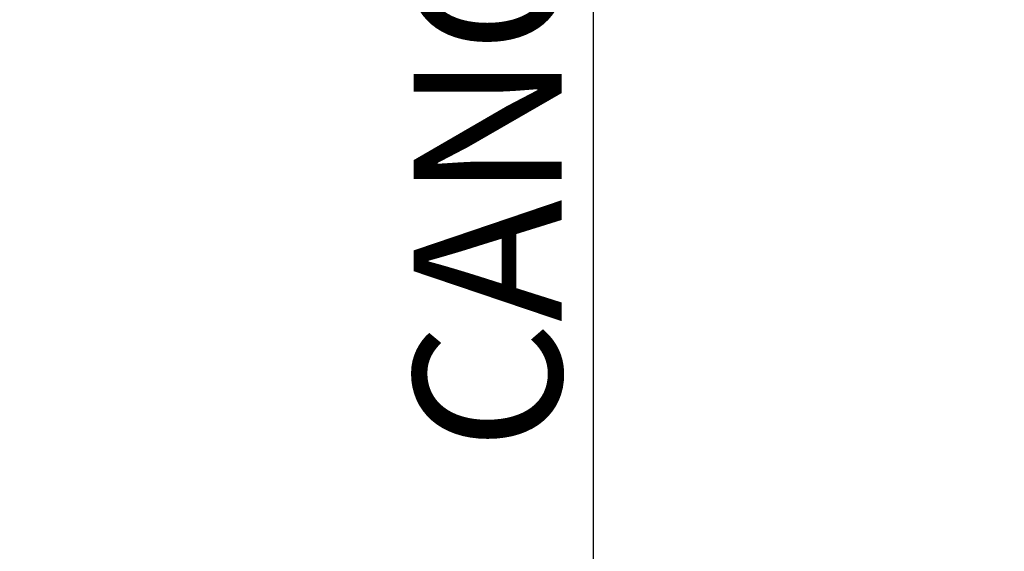
# Model space of a CAD drawing. Units: millimetres. Extents: x 595116 to 630915, y 909473 to 920225.
# Tile 65 of 134: x 629559 to 629619, y 919314 to 919346. Entities that reach past the tile are written whole.
import ezdxf

# ---------------------------------------------------------------- set-up
doc = ezdxf.new("R2010")
doc.units = ezdxf.units.MM
doc.layers.add('Dimension', color=3, linetype='Continuous', lineweight=18)
doc.styles.get("Standard").update_dxf_attribs({"font": 'arial.ttf'})
doc.dimstyles.new('ISO-25', dxfattribs={"dimtxt": 9, "dimasz": 6, "dimexe": 1.25, "dimexo": 0.625, "dimtad": 1, "dimlunit": 4, "dimtxsty": 'Standard', "dimcen": 2.5, "dimadec": 0, "dimazin": 0, "dimtfac": 1, "dimtmove": 0, "dimatfit": 3, "dimfxl": 1, "dimarcsym": 0})

# ---------------------------------------------------------------- blocks, each defined once
blk = doc.blocks.new('*D210')
at = {"layer": 'Defpoints', "color": 0, "transparency": 16777216}
for p in [(629586.227, 919310.123), (629593.946, 919310.123), (629586.227, 919258.662)]:
    blk.add_point(p, dxfattribs=at)
at = {"layer": 'Dimension', "color": 0, "lineweight": -2, "transparency": 16777216}
for p, q in [((629593.946, 919310.123), (629593.946, 919449.69)), ((629586.852, 919310.123), (629595.196, 919310.123)), ((629593.946, 919264.662), (629593.946, 919304.123)), ((629586.852, 919258.662), (629595.196, 919258.662))]:
    blk.add_line(p, q, dxfattribs=at)
at = {"layer": 'Dimension', "color": 0, "transparency": 16777216}
for points in [[(629592.946, 919304.123), (629594.946, 919304.123), (629593.946, 919310.123)], [(629592.946, 919264.662), (629594.946, 919264.662), (629593.946, 919258.662)]]:
    blk.add_solid(points, dxfattribs=at)
at = {"layer": 'Dimension', "color": 0, "transparency": 16777216, "insert": (629588.662, 919382.907), "char_height": 9, "attachment_point": 5, "rotation": 90}
blk.add_mtext('CANOPY 4\'-3 1/2" TYP.', dxfattribs=at)
blk = doc.blocks.new('*D216')
at = {"layer": 'Defpoints', "color": 0, "transparency": 16777216}
for p in [(629505.041, 919411.828), (629743.541, 919411.928), (629743.541, 918832.378)]:
    blk.add_point(p, dxfattribs=at)
at = {"layer": 'Dimension', "color": 0, "lineweight": -2, "transparency": 16777216}
for p, q in [((629505.041, 919411.203), (629505.041, 918831.128)), ((629743.541, 919411.303), (629743.541, 918831.128)), ((629511.041, 918832.378), (629737.541, 918832.378))]:
    blk.add_line(p, q, dxfattribs=at)
at = {"layer": 'Dimension', "color": 0, "transparency": 16777216}
for points in [[(629511.041, 918833.378), (629511.041, 918831.378), (629505.041, 918832.378)], [(629737.541, 918833.378), (629737.541, 918831.378), (629743.541, 918832.378)]]:
    blk.add_solid(points, dxfattribs=at)
at = {"layer": 'Dimension', "color": 0, "transparency": 16777216, "insert": (629624.291, 918837.656), "char_height": 9, "attachment_point": 5}
blk.add_mtext('19\'-10 1/2"', dxfattribs=at)
blk = doc.blocks.new('*D220')
at = {"layer": 'Defpoints', "color": 0, "transparency": 16777216}
for p in [(629824.951, 920160.756), (629511.274, 919302.009), (629824.951, 919302.009)]:
    blk.add_point(p, dxfattribs=at)
at = {"layer": 'Dimension', "color": 0, "lineweight": -2, "transparency": 16777216}
for p, q in [((629511.274, 919302.634), (629511.274, 920162.006)), ((629824.951, 919302.634), (629824.951, 920162.006)), ((629517.274, 920160.756), (629818.951, 920160.756))]:
    blk.add_line(p, q, dxfattribs=at)
at = {"layer": 'Dimension', "color": 0, "transparency": 16777216}
for points in [[(629517.274, 920161.756), (629517.274, 920159.756), (629511.274, 920160.756)], [(629818.951, 920161.756), (629818.951, 920159.756), (629824.951, 920160.756)]]:
    blk.add_solid(points, dxfattribs=at)
at = {"layer": 'Dimension', "color": 0, "transparency": 16777216, "insert": (629668.113, 920166.035), "char_height": 9, "attachment_point": 5}
blk.add_mtext('26\'-1 1/2"', dxfattribs=at)

msp = doc.modelspace()

# ---------------------------------------------------------------- dimensions: what is measured, and where the dimension line sits
at = {"layer": 'Dimension'}
for base, p1, p2, picture, middle in [((629824.951, 920160.756), (629511.274, 919302.009), (629824.951, 919302.009), '*D220', (629668.113, 920166.035)), ((629743.541, 918832.378), (629505.041, 919411.828), (629743.541, 919411.928), '*D216', (629624.291, 918837.656))]:
    dim = msp.add_linear_dim(base=base, p1=p1, p2=p2, dimstyle='ISO-25', override={"dimdec": 1, "dimlfac": 1, "dimrnd": 0, "dimzin": 1, "dimdsep": 46, "dimlunit": 4, "dimfrac": 2}, dxfattribs=at)
    dim.commit()
    dim.dimension.update_dxf_attribs({"geometry": picture, "text_midpoint": middle})
dim = msp.add_linear_dim(base=(629593.946, 919310.123), p1=(629586.227, 919258.662), p2=(629586.227, 919310.123), angle=90, text='CANOPY <> TYP.', dimstyle='ISO-25', override={"dimdec": 1, "dimlfac": 1, "dimrnd": 0, "dimzin": 1, "dimdsep": 46, "dimlunit": 4, "dimfrac": 2}, dxfattribs=at)
dim.commit()
dim.dimension.update_dxf_attribs({"geometry": '*D210', "text_midpoint": (629588.662, 919382.907)})

doc.saveas('drawing.dxf')
